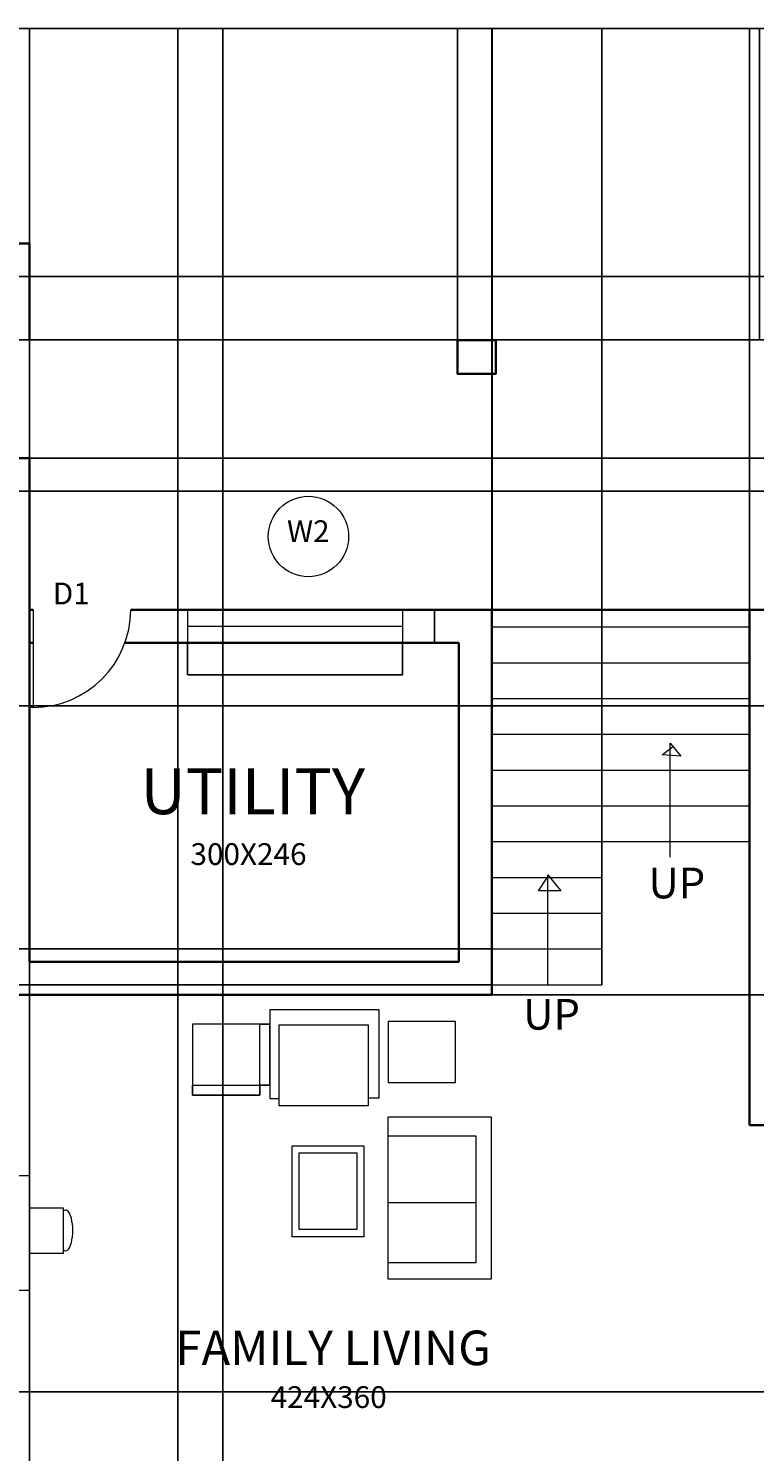
# Model space of a CAD drawing. Units: millimetres. Extents: x -2968 to 14333, y -2966 to 13411.
# Tile 2 of 3: x 3229 to 8301, y 3466 to 13411. Entities that reach past the tile are written whole.
import ezdxf

# ---------------------------------------------------------------- set-up
doc = ezdxf.new("R2010")
doc.units = ezdxf.units.MM
doc.header["$MEASUREMENT"] = 0
for name, color, linetype, lineweight in [('A-ANNO-DIMS', 2, 'Continuous', 18), ('A-ANNO-SYMB', 3, 'Continuous', 13), ('A-ANNO-TEXT', 7, 'Continuous', 18), ('A-AREA-IDEN', 7, 'Continuous', 18), ('A-COLS', 7, 'Continuous', 35), ('A-DOOR', 3, 'Continuous', 18), ('A-FLOR-EDGE', 7, 'Continuous', 25), ('A-FLOR-STRS', 7, 'Continuous', 18), ('A-FURN', 8, 'Continuous', 18), ('A-GLAZ', 4, 'Continuous', 18), ('A-WALL', 7, 'Continuous', 35)]:
    doc.layers.add(name, color=color, linetype=linetype, lineweight=lineweight)
doc.styles.get("Standard").update_dxf_attribs({"font": 'arial.ttf'})
doc.dimstyles.get("Standard").update_dxf_attribs({"dimtxt": 0.18, "dimasz": 0.18, "dimexe": 0.18, "dimexo": 0.0625, "dimgap": 0.09, "dimtad": 0, "dimtih": 1, "dimtoh": 1, "dimdec": 4, "dimzin": 0, "dimdsep": 46, "dimtxsty": 'Standard', "dimcen": 0.09, "dimadec": 0, "dimazin": 0, "dimtfac": 1, "dimtdec": 4, "dimtofl": 0, "dimtmove": 0, "dimatfit": 3, "dimfxl": 1, "dimtolj": 1, "dimtzin": 0, "dimarcsym": 0})

# ---------------------------------------------------------------- blocks, each defined once
blk = doc.blocks.new('WIN-1500')
for p, q in [((-0.0001454069465439, 230.0001364428754), (-0.0001454069465439, 0.0001364428753732)), ((1499.999854593053, 230.0001364428754), (1499.999854593053, 0.0001364428753732)), ((-0.0001454069465439, 115.0001364428753), (1499.999854593053, 115.0001364428753))]:
    blk.add_line(p, q)
blk = doc.blocks.new('DINING-CHAIR')
blk.add_lwpolyline([(8.40971169964e-05, 318.4642751495176), (234.8798944680875, 318.4642751495176), (234.8798944680875, -0.0002547686981416), (8.40971169964e-05, -0.0002547686981416)], close=True)
blk.add_ellipse((251.6572223520761, 161.1385219065178), major_axis=(0, 142.4711695614969), ratio=0.3529417904011299, start_param=2.801418553469442, end_param=6.623359407299936)
blk = doc.blocks.new('VERANDAH-POST')
blk.add_lwpolyline([(-5.84108229305e-05, 235.3216454025205), (266.2404368537072, 235.3216454025205), (266.2404368537072, -0.0003482651118247), (-5.84108229305e-05, -0.0003482651118247)], close=True)
blk = doc.blocks.new('END-TABLE')
blk.add_lwpolyline([(470.3905178718432, 425.6120167429653), (-0.0001639190431888, 425.6120167429653), (-0.0001639190431888, -0.0003055184752156), (470.3905178718432, -0.0003055184752156)], close=True)
blk = doc.blocks.new('*D16')
at = {"layer": 'A-ANNO-DIMS', "color": 0, "lineweight": -2, "transparency": 16777216}
for p, q in [((4341.04331944906, 9117.637743151285), (4341.04331944906, 8892.520243151284)), ((5841.04331944906, 9117.637743151285), (5841.04331944906, 8892.520243151284)), ((4341.223319449061, 8892.700243151285), (5089.785099803767, 8892.700243151285)), ((5840.863319449059, 8892.700243151285), (5092.301539094354, 8892.700243151285))]:
    blk.add_line(p, q, dxfattribs=at)
at = {"layer": 'A-ANNO-DIMS', "color": 0, "transparency": 16777216}
for points in [[(4341.223319449061, 8892.730243151285), (4341.223319449061, 8892.670243151284), (4341.04331944906, 8892.700243151285)], [(5840.863319449059, 8892.730243151285), (5840.863319449059, 8892.670243151284), (5841.04331944906, 8892.700243151285)]]:
    blk.add_solid(points, dxfattribs=at)
at = {"layer": 'Defpoints', "color": 0, "transparency": 16777216}
for p in [(4341.04331944906, 9117.700243151285), (5841.04331944906, 9117.700243151285), (5841.04331944906, 8892.700243151285)]:
    blk.add_point(p, dxfattribs=at)
at = {"layer": 'A-ANNO-DIMS', "color": 0, "transparency": 16777216, "insert": (5091.04331944906, 8892.700243151285), "char_height": 0.18, "attachment_point": 5}
blk.add_mtext('\\A1;WINDOW 1500 TYP.', dxfattribs=at)
blk = doc.blocks.new('*D17')
at = {"layer": 'A-ANNO-DIMS', "color": 0, "lineweight": -2, "transparency": 16777216}
for p, q in [((5841.105819449062, 9347.700243151288), (6066.223319449064, 9347.700243151288)), ((6066.043319449064, 9347.520243151288), (6066.043319449064, 9232.88220768062)), ((6066.043319449064, 9117.880243151289), (6066.043319449064, 9232.518278621958)), ((5841.105819449062, 9117.700243151288), (6066.223319449064, 9117.700243151288))]:
    blk.add_line(p, q, dxfattribs=at)
at = {"layer": 'A-ANNO-DIMS', "color": 0, "transparency": 16777216}
for points in [[(6066.013319449064, 9347.520243151288), (6066.073319449063, 9347.520243151288), (6066.043319449064, 9347.700243151288)], [(6066.013319449064, 9117.880243151289), (6066.073319449063, 9117.880243151289), (6066.043319449064, 9117.700243151288)]]:
    blk.add_solid(points, dxfattribs=at)
at = {"layer": 'Defpoints', "color": 0, "transparency": 16777216}
for p in [(5841.043319449061, 9347.700243151288), (6066.043319449064, 9347.700243151288), (5841.043319449061, 9117.700243151288)]:
    blk.add_point(p, dxfattribs=at)
at = {"layer": 'A-ANNO-DIMS', "color": 0, "transparency": 16777216, "insert": (6066.043319449065, 9232.700243151285), "char_height": 0.18, "attachment_point": 5}
blk.add_mtext('\\A1;230 TYP.', dxfattribs=at)
blk = doc.blocks.new('*D22')
at = {"layer": 'A-ANNO-DIMS', "color": 0, "lineweight": -2, "transparency": 16777216}
for p, q in [((4375.117836080957, 6026.510194481525), (4375.117836080957, 5955.834092212892)), ((4845.508517871843, 6026.510194481525), (4845.508517871843, 5955.834092212892)), ((4375.297836080958, 5956.014092212893), (4608.986260196046, 5956.014092212893)), ((4845.328517871843, 5956.014092212893), (4611.640093756755, 5956.014092212893))]:
    blk.add_line(p, q, dxfattribs=at)
at = {"layer": 'A-ANNO-DIMS', "color": 0, "transparency": 16777216}
for points in [[(4375.297836080958, 5956.044092212891), (4375.297836080958, 5955.984092212893), (4375.117836080957, 5956.014092212893)], [(4845.328517871843, 5956.044092212891), (4845.328517871843, 5955.984092212893), (4845.508517871843, 5956.014092212893)]]:
    blk.add_solid(points, dxfattribs=at)
at = {"layer": 'Defpoints', "color": 0, "transparency": 16777216}
for p in [(4375.117836080957, 6026.572694481525), (4845.508517871843, 6026.572694481525), (4845.508517871843, 5956.014092212893)]:
    blk.add_point(p, dxfattribs=at)
at = {"layer": 'A-ANNO-DIMS', "color": 0, "transparency": 16777216, "insert": (4610.3131769764, 5956.014092212893), "char_height": 0.18, "attachment_point": 5}
blk.add_mtext('\\A1;END TABLE 470 TYP.', dxfattribs=at)
blk = doc.blocks.new('*D23')
at = {"layer": 'A-ANNO-DIMS', "color": 0, "lineweight": -2, "transparency": 16777216}
for p, q in [((4845.571017871845, 6452.185016742969), (4916.24712014048, 6452.185016742969)), ((4916.06712014048, 6452.005016742969), (4916.06712014048, 6239.560758750037)), ((4916.067120140481, 6026.752694481527), (4916.06712014048, 6239.196952474458)), ((4845.571017871845, 6026.572694481527), (4916.247120140481, 6026.572694481527))]:
    blk.add_line(p, q, dxfattribs=at)
at = {"layer": 'A-ANNO-DIMS', "color": 0, "transparency": 16777216}
for points in [[(4916.03712014048, 6452.005016742969), (4916.09712014048, 6452.005016742969), (4916.06712014048, 6452.185016742969)], [(4916.037120140481, 6026.752694481527), (4916.097120140481, 6026.752694481527), (4916.067120140481, 6026.572694481527)]]:
    blk.add_solid(points, dxfattribs=at)
at = {"layer": 'Defpoints', "color": 0, "transparency": 16777216}
for p in [(4845.508517871845, 6452.185016742969), (4916.06712014048, 6452.185016742969), (4845.508517871845, 6026.572694481527)]:
    blk.add_point(p, dxfattribs=at)
at = {"layer": 'A-ANNO-DIMS', "color": 0, "transparency": 16777216, "insert": (4916.067120140481, 6239.378855612245), "char_height": 0.18, "attachment_point": 5}
blk.add_mtext('\\A1;426 TYP.', dxfattribs=at)
blk = doc.blocks.new('*D32')
at = {"layer": 'A-ANNO-DIMS', "color": 0, "lineweight": -2, "transparency": 16777216}
for p, q in [((-1494.810979, 11907.569973), (-1494.810979, 13410.507299)), ((-1494.630979, 13410.327299), (5659.769102855388, 13410.327299)), ((12815.009021, 13410.327299), (5660.608939144611, 13410.327299)), ((12815.189021, 11235.596939), (12815.189021, 13410.507299))]:
    blk.add_line(p, q, dxfattribs=at)
at = {"layer": 'A-ANNO-DIMS', "color": 0, "transparency": 16777216}
for points in [[(-1494.630979, 13410.357299), (-1494.630979, 13410.297299), (-1494.810979, 13410.327299)], [(12815.009021, 13410.357299), (12815.009021, 13410.297299), (12815.189021, 13410.327299)]]:
    blk.add_solid(points, dxfattribs=at)
at = {"layer": 'Defpoints', "color": 0, "transparency": 16777216}
for p in [(12815.189021, 13410.327299), (-1494.810979, 11907.507473), (12815.189021, 11235.534439)]:
    blk.add_point(p, dxfattribs=at)
at = {"layer": 'A-ANNO-DIMS', "color": 0, "transparency": 16777216, "insert": (5660.189021, 13410.327299), "char_height": 0.18, "attachment_point": 5}
blk.add_mtext('\\A1;14310', dxfattribs=at)
blk = doc.blocks.new('*D43')
at = {"layer": 'A-ANNO-DIMS', "color": 0, "lineweight": -2, "transparency": 16777216}
for p, q in [((6465.189021, 9347.569973), (6465.189021, 13410.507299)), ((6465.369021, 13410.327299), (7364.839027821282, 13410.327299)), ((8265.009021, 13410.327299), (7365.539014178718, 13410.327299)), ((8265.189021, 9347.569973), (8265.189021, 13410.507299))]:
    blk.add_line(p, q, dxfattribs=at)
at = {"layer": 'A-ANNO-DIMS', "color": 0, "transparency": 16777216}
for points in [[(6465.369021, 13410.357299), (6465.369021, 13410.297299), (6465.189021, 13410.327299)], [(8265.009021, 13410.357299), (8265.009021, 13410.297299), (8265.189021, 13410.327299)]]:
    blk.add_solid(points, dxfattribs=at)
at = {"layer": 'Defpoints', "color": 0, "transparency": 16777216}
for p in [(8265.189021, 13410.327299), (6465.189021, 9347.507473), (8265.189021, 9347.507473)]:
    blk.add_point(p, dxfattribs=at)
at = {"layer": 'A-ANNO-DIMS', "color": 0, "transparency": 16777216, "insert": (7365.189021, 13410.327299), "char_height": 0.18, "attachment_point": 5}
blk.add_mtext('\\A1;1800', dxfattribs=at)
blk = doc.blocks.new('*D44')
at = {"layer": 'A-ANNO-DIMS', "color": 0, "lineweight": -2, "transparency": 16777216}
for p, q in [((6467.365993, 6728.435381999999), (6467.365993, 13410.507299)), ((6467.545993, 13410.327299), (6850.884355567531, 13410.327299)), ((7235.009021, 13410.327299), (6851.670658432471, 13410.327299)), ((7235.189021, 6728.435381999999), (7235.189021, 13410.507299))]:
    blk.add_line(p, q, dxfattribs=at)
at = {"layer": 'A-ANNO-DIMS', "color": 0, "transparency": 16777216}
for points in [[(6467.545993, 13410.357299), (6467.545993, 13410.297299), (6467.365993, 13410.327299)], [(7235.009021, 13410.357299), (7235.009021, 13410.297299), (7235.189021, 13410.327299)]]:
    blk.add_solid(points, dxfattribs=at)
at = {"layer": 'Defpoints', "color": 0, "transparency": 16777216}
for p in [(7235.189021, 13410.327299), (6467.365993, 6728.372881999999), (7235.189021, 6728.372881999999)]:
    blk.add_point(p, dxfattribs=at)
at = {"layer": 'A-ANNO-DIMS', "color": 0, "transparency": 16777216, "insert": (6851.277507, 13410.327299), "char_height": 0.18, "attachment_point": 5}
blk.add_mtext('\\A1;767.8', dxfattribs=at)
blk = doc.blocks.new('*D45')
at = {"layer": 'A-ANNO-DIMS', "color": 0, "lineweight": -2, "transparency": 16777216}
for p, q in [((6467.303493000004, 6978.372882000003), (-2967.835419000002, 6978.372882000002)), ((-2967.655419000002, 6978.192882000001), (-2967.655419000002, 6853.554785137792)), ((-2967.655419000002, 6728.552882000002), (-2967.655419000002, 6853.190978862212)), ((6467.303493000004, 6728.372882000003), (-2967.835419000002, 6728.372882000002))]:
    blk.add_line(p, q, dxfattribs=at)
at = {"layer": 'A-ANNO-DIMS', "color": 0, "transparency": 16777216}
for points in [[(-2967.685419000002, 6978.192882000001), (-2967.625419000002, 6978.192882000001), (-2967.655419000002, 6978.372882000002)], [(-2967.685419000002, 6728.552882000002), (-2967.625419000002, 6728.552882000002), (-2967.655419000002, 6728.372882000002)]]:
    blk.add_solid(points, dxfattribs=at)
at = {"layer": 'Defpoints', "color": 0, "transparency": 16777216}
for p in [(-2967.655419000002, 6978.372882000002), (6467.365993000004, 6978.372882000003), (6467.365993000004, 6728.372882000003)]:
    blk.add_point(p, dxfattribs=at)
at = {"layer": 'A-ANNO-DIMS', "color": 0, "transparency": 16777216, "insert": (-2967.655419, 6853.372882000001), "char_height": 0.18, "attachment_point": 5}
blk.add_mtext('\\A1;250', dxfattribs=at)
blk = doc.blocks.new('*D47')
at = {"layer": 'A-ANNO-DIMS', "color": 0, "lineweight": -2, "transparency": 16777216}
for p, q in [((-1264.748479, 11677.507473), (14333.28935600001, 11677.507473)), ((14333.10935600001, 11677.327473), (14333.10935600001, 11042.68937613779)), ((14333.10935600001, 10407.687473), (14333.10935600001, 11042.32556986221)), ((-1264.748479, 10407.507473), (14333.28935600001, 10407.507473))]:
    blk.add_line(p, q, dxfattribs=at)
at = {"layer": 'A-ANNO-DIMS', "color": 0, "transparency": 16777216}
for points in [[(14333.07935600001, 11677.327473), (14333.13935600001, 11677.327473), (14333.10935600001, 11677.507473)], [(14333.07935600001, 10407.687473), (14333.13935600001, 10407.687473), (14333.10935600001, 10407.507473)]]:
    blk.add_solid(points, dxfattribs=at)
at = {"layer": 'Defpoints', "color": 0, "transparency": 16777216}
for p in [(-1264.810979000001, 11677.507473), (14333.10935600001, 11677.507473), (-1264.810979000001, 10407.507473)]:
    blk.add_point(p, dxfattribs=at)
at = {"layer": 'A-ANNO-DIMS', "color": 0, "transparency": 16777216, "insert": (14333.10935600001, 11042.507473), "char_height": 0.18, "attachment_point": 5}
blk.add_mtext('\\A1;1270', dxfattribs=at)
blk = doc.blocks.new('*D49')
at = {"layer": 'A-ANNO-DIMS', "color": 0, "lineweight": -2, "transparency": 16777216}
for p, q in [((3235.189021, 232.569973), (3235.189021000001, 13410.507299)), ((3235.369021000001, 13410.327299), (3753.817212416781, 13410.327299)), ((4273.14097, 13410.327299), (3754.69277858322, 13410.327299)), ((4273.320969999999, 232.569973), (4273.320970000001, 13410.507299))]:
    blk.add_line(p, q, dxfattribs=at)
at = {"layer": 'A-ANNO-DIMS', "color": 0, "transparency": 16777216}
for points in [[(3235.369021000001, 13410.357299), (3235.369021000001, 13410.297299), (3235.189021000001, 13410.327299)], [(4273.14097, 13410.357299), (4273.14097, 13410.297299), (4273.320970000001, 13410.327299)]]:
    blk.add_solid(points, dxfattribs=at)
at = {"layer": 'Defpoints', "color": 0, "transparency": 16777216}
for p in [(4273.320970000001, 13410.327299), (3235.189021, 232.507473), (4273.320969999999, 232.507473)]:
    blk.add_point(p, dxfattribs=at)
at = {"layer": 'A-ANNO-DIMS', "color": 0, "transparency": 16777216, "insert": (3754.254995500001, 13410.327299), "char_height": 0.18, "attachment_point": 5}
blk.add_mtext('\\A1;1038.1', dxfattribs=at)
blk = doc.blocks.new('*D50')
at = {"layer": 'A-ANNO-DIMS', "color": 0, "lineweight": -2, "transparency": 16777216}
for p, q in [((3235.189021, 11235.596939), (3235.189021, 13410.507299)), ((3235.369021, 13410.327299), (4730.825595415415, 13410.327299)), ((6227.000942, 13410.327299), (4731.544367584583, 13410.327299)), ((6227.180942, 11232.243145), (6227.180942, 13410.507299))]:
    blk.add_line(p, q, dxfattribs=at)
at = {"layer": 'A-ANNO-DIMS', "color": 0, "transparency": 16777216}
for points in [[(3235.369021, 13410.357299), (3235.369021, 13410.297299), (3235.189021, 13410.327299)], [(6227.000942, 13410.357299), (6227.000942, 13410.297299), (6227.180942, 13410.327299)]]:
    blk.add_solid(points, dxfattribs=at)
at = {"layer": 'Defpoints', "color": 0, "transparency": 16777216}
for p in [(6227.180942, 13410.327299), (3235.189021, 11235.534439), (6227.180942, 11232.180645)]:
    blk.add_point(p, dxfattribs=at)
at = {"layer": 'A-ANNO-DIMS', "color": 0, "transparency": 16777216, "insert": (4731.184981499999, 13410.327299), "char_height": 0.18, "attachment_point": 5}
blk.add_mtext('\\A1;2992', dxfattribs=at)
blk = doc.blocks.new('*D51')
at = {"layer": 'A-ANNO-DIMS', "color": 0, "lineweight": -2, "transparency": 16777216}
for p, q in [((6227.180942, 11232.243145), (6227.180942, 13410.507299)), ((6227.360942, 13410.327299), (7281.505338680763, 13410.327299)), ((8336.57994, 13410.327299), (7282.435543319237, 13410.327299)), ((8336.75994, 11232.243145), (8336.75994, 13410.507299))]:
    blk.add_line(p, q, dxfattribs=at)
at = {"layer": 'A-ANNO-DIMS', "color": 0, "transparency": 16777216}
for points in [[(6227.360942, 13410.357299), (6227.360942, 13410.297299), (6227.180942, 13410.327299)], [(8336.57994, 13410.357299), (8336.57994, 13410.297299), (8336.75994, 13410.327299)]]:
    blk.add_solid(points, dxfattribs=at)
at = {"layer": 'Defpoints', "color": 0, "transparency": 16777216}
for p in [(8336.75994, 13410.327299), (6227.180942, 11232.180645), (8336.75994, 11232.180645)]:
    blk.add_point(p, dxfattribs=at)
at = {"layer": 'A-ANNO-DIMS', "color": 0, "transparency": 16777216, "insert": (7281.970441, 13410.327299), "char_height": 0.18, "attachment_point": 5}
blk.add_mtext('\\A1;2109.6', dxfattribs=at)
blk = doc.blocks.new('*D54')
at = {"layer": 'A-ANNO-DIMS', "color": 0, "lineweight": -2, "transparency": 16777216}
for p, q in [((-1220.345468, 3884.149375000002), (14333.28935600001, 3884.149375000005)), ((14333.10935600001, 3883.969375000005), (14333.10935600001, 2738.596660637794)), ((14333.10935600001, 1592.860140000003), (14333.10935600001, 2738.232854362214)), ((-1220.345468, 1592.680140000001), (14333.28935600001, 1592.680140000003))]:
    blk.add_line(p, q, dxfattribs=at)
at = {"layer": 'A-ANNO-DIMS', "color": 0, "transparency": 16777216}
for points in [[(14333.07935600001, 3883.969375000005), (14333.13935600001, 3883.969375000005), (14333.10935600001, 3884.149375000005)], [(14333.07935600001, 1592.860140000003), (14333.13935600001, 1592.860140000003), (14333.10935600001, 1592.680140000003)]]:
    blk.add_solid(points, dxfattribs=at)
at = {"layer": 'Defpoints', "color": 0, "transparency": 16777216}
for p in [(-1220.407968, 3884.149375000002), (14333.10935600001, 3884.149375000005), (-1220.407968, 1592.680140000001)]:
    blk.add_point(p, dxfattribs=at)
at = {"layer": 'A-ANNO-DIMS', "color": 0, "transparency": 16777216, "insert": (14333.10935600001, 2738.414757499999), "char_height": 0.18, "attachment_point": 5}
blk.add_mtext('\\A1;2291.5', dxfattribs=at)
blk = doc.blocks.new('*D55')
at = {"layer": 'A-ANNO-DIMS', "color": 0, "lineweight": -2, "transparency": 16777216}
for p, q in [((-1494.748479, 6657.507473000004), (14333.28935600001, 6657.507473000006)), ((14333.10935600001, 6657.327473000005), (14333.10935600001, 5271.010388529336)), ((14333.10935600002, 3884.329375000005), (14333.10935600001, 5270.646459470672)), ((-1220.345468, 3884.149375000002), (14333.28935600002, 3884.149375000005))]:
    blk.add_line(p, q, dxfattribs=at)
at = {"layer": 'A-ANNO-DIMS', "color": 0, "transparency": 16777216}
for points in [[(14333.07935600001, 6657.327473000005), (14333.13935600001, 6657.327473000005), (14333.10935600001, 6657.507473000006)], [(14333.07935600002, 3884.329375000005), (14333.13935600001, 3884.329375000005), (14333.10935600002, 3884.149375000005)]]:
    blk.add_solid(points, dxfattribs=at)
at = {"layer": 'Defpoints', "color": 0, "transparency": 16777216}
for p in [(-1494.810979, 6657.507473000004), (14333.10935600001, 6657.507473000006), (-1220.407968, 3884.149375000002)]:
    blk.add_point(p, dxfattribs=at)
at = {"layer": 'A-ANNO-DIMS', "color": 0, "transparency": 16777216, "insert": (14333.10935600001, 5270.828424), "char_height": 0.18, "attachment_point": 5}
blk.add_mtext('\\A1;2773.4', dxfattribs=at)
blk = doc.blocks.new('*D57')
at = {"layer": 'A-ANNO-DIMS', "color": 0, "lineweight": -2, "transparency": 16777216}
for p, q in [((1665.064982, -1259.254558), (1665.064982000001, 13410.507299)), ((1665.244982000001, 13410.327299), (3125.078715848568, 13410.327299)), ((4585.598316000001, 13410.327299), (3125.764582151433, 13410.327299)), ((4585.778315999999, -1259.254558), (4585.778316000001, 13410.507299))]:
    blk.add_line(p, q, dxfattribs=at)
at = {"layer": 'A-ANNO-DIMS', "color": 0, "transparency": 16777216}
for points in [[(1665.244982000001, 13410.357299), (1665.244982000001, 13410.297299), (1665.064982000001, 13410.327299)], [(4585.598316000001, 13410.357299), (4585.598316000001, 13410.297299), (4585.778316000001, 13410.327299)]]:
    blk.add_solid(points, dxfattribs=at)
at = {"layer": 'Defpoints', "color": 0, "transparency": 16777216}
for p in [(4585.778316000001, 13410.327299), (1665.064982, -1259.317058), (4585.778315999999, -1259.317058)]:
    blk.add_point(p, dxfattribs=at)
at = {"layer": 'A-ANNO-DIMS', "color": 0, "transparency": 16777216, "insert": (3125.421649000001, 13410.327299), "char_height": 0.18, "attachment_point": 5}
blk.add_mtext('\\A1;2921', dxfattribs=at)
blk = doc.blocks.new('*D61')
at = {"layer": 'A-ANNO-DIMS', "color": 0, "lineweight": -2, "transparency": 16777216}
for p, q in [((1505.251521, 10177.507473), (14333.28935600001, 10177.507473)), ((14333.10935600001, 10177.327473), (14333.10935600001, 9427.689376137798)), ((14333.10935600001, 8677.687473000007), (14333.10935600001, 9427.325569862218)), ((1505.251521, 8677.507473000003), (14333.28935600001, 8677.507473000007))]:
    blk.add_line(p, q, dxfattribs=at)
at = {"layer": 'A-ANNO-DIMS', "color": 0, "transparency": 16777216}
for points in [[(14333.07935600001, 10177.327473), (14333.13935600001, 10177.327473), (14333.10935600001, 10177.507473)], [(14333.07935600001, 8677.687473000007), (14333.13935600001, 8677.687473000007), (14333.10935600001, 8677.507473000007)]]:
    blk.add_solid(points, dxfattribs=at)
at = {"layer": 'Defpoints', "color": 0, "transparency": 16777216}
for p in [(1505.189021, 10177.507473), (14333.10935600001, 10177.507473), (1505.189021, 8677.507473000003)]:
    blk.add_point(p, dxfattribs=at)
at = {"layer": 'A-ANNO-DIMS', "color": 0, "transparency": 16777216, "insert": (14333.10935600001, 9427.507473000001), "char_height": 0.18, "attachment_point": 5}
blk.add_mtext('\\A1;1500', dxfattribs=at)

msp = doc.modelspace()

# ---------------------------------------------------------------- linework, layer by layer
at = {"layer": 'A-ANNO-SYMB'}
for points in [[(7712.199242320145, 7618.934004650917), (7712.199242320145, 8415.524808817892), (7785.424564020941, 8326.111813228461), (7655.246677664807, 8334.240447608754), (7728.471999365604, 8391.13940132549)], [(6857.902432476404, 6732.929709246033), (6857.902432476404, 7497.006967188733), (6947.400511222426, 7383.208068458421), (6792.812794297235, 7383.208068458421), (6849.765358952573, 7472.621559696271)]]:
    msp.add_lwpolyline(points, dxfattribs=at)
msp.add_circle((5184.743742056191, 9860.213910516351), 280.7929963504647, dxfattribs=at)
at = {"layer": 'A-DOOR'}
msp.add_lwpolyline([(3261.29201869457, 9347.836903303887), (3261.29201869457, 8666.348579443365), (3233.993676473896, 8666.348579443365), (3233.993676473896, 9347.836903303887)], close=True, dxfattribs=at)
msp.add_arc((3261.29201869457, 9347.836903303887), 681.7287306783696, 270, 0, dxfattribs=at)
at = {"layer": 'A-FLOR-EDGE'}
msp.add_line((3005.189021442665, 11235.53443915362), (12815.18902144266, 11235.53443915362), dxfattribs=at)
at = {"layer": 'A-FLOR-STRS'}
for p, q in [((7235.189021442668, 6728.372881745513), (7235.189021442664, 9347.507473364632)), ((6467.365993403596, 9228.372881745512), (8265.45908183977, 9228.372881745512)), ((6467.365993403596, 8978.372881745512), (8265.45908183977, 8978.372881745512)), ((6467.365993403596, 8728.372881745512), (8265.45908183977, 8728.372881745512)), ((6467.365993403596, 8478.372881745512), (8265.45908183977, 8478.372881745512)), ((6467.365993403596, 8228.372881745512), (8265.45908183977, 8228.372881745512)), ((6467.365993403596, 7978.372881745513), (8265.45908183977, 7978.372881745513)), ((6467.365993403596, 7728.372881745513), (8265.45908183977, 7728.372881745513)), ((6467.365993403596, 7478.372881745513), (7235.189021442668, 7478.372881745513)), ((8265.189021442662, 7478.372881745513), (8265.45908183977, 7478.372881745513)), ((6467.365993403596, 7228.372881745513), (7235.189021442668, 7228.372881745513)), ((8265.189021442662, 7228.372881745513), (8265.45908183977, 7228.372881745513)), ((6467.365993403596, 6978.372881745513), (7235.189021442668, 6978.372881745513)), ((8265.189021442662, 6978.372881745513), (8265.45908183977, 6978.372881745513)), ((6467.365993403596, 6728.372881745513), (7235.189021442668, 6728.372881745513)), ((8265.189021442662, 6728.372881745511), (8265.45908183977, 6728.372881745513))]:
    msp.add_line(p, q, dxfattribs=at)
at = {"layer": 'A-FURN'}
msp.add_line((5741.930737728253, 5207.03832412773), (6355.116356844548, 5207.03832412773), dxfattribs=at)
for points in [[(5602.331415713532, 5937.838241603458), (5679.990844783839, 5937.838241603458), (5679.990844783839, 6552.981074355485), (4914.495722528547, 6552.981074355485), (4914.495722528547, 5932.296396420163), (4981.060153158847, 5932.296396420163)], [(5741.915447702631, 5671.896089695977), (6354.311545506818, 5671.896089695977), (6354.311545506818, 4785.203834259358), (5741.915447702631, 4785.203834259358)]]:
    msp.add_lwpolyline(points, dxfattribs=at)
for points in [[(4981.060153158847, 6447.686511521286), (5602.331415713532, 6447.686511521286), (5602.331415713532, 5882.420285418921), (4981.060153158847, 5882.420285418921)], [(5741.915447702631, 5804.899878446595), (6460.814912515693, 5804.899878446595), (6460.814912515693, 4669.933850965579), (5741.915447702631, 4669.933850965579)], [(5070.613831997383, 5602.638637830562), (5572.326825845987, 5602.638637830562), (5572.326825845987, 4966.451068057039), (5070.613831997383, 4966.451068057039)], [(5120.613831997383, 5552.638637830561), (5522.326825845986, 5552.638637830561), (5522.326825845986, 5016.451068057039), (5120.613831997383, 5016.451068057039)], [(627.8926181816496, 5394.823160820234), (3236.742084097117, 5394.823160820234), (3236.742084097117, 4590.28017311683), (627.8926181816496, 4590.28017311683)]]:
    msp.add_lwpolyline(points, close=True, dxfattribs=at)
at = {"layer": 'A-WALL'}
for p, q in [((-1494.810978557335, 11907.50747336463), (3235.189021442665, 11907.50747336463)), ((3235.189021442665, 11235.53443915362), (3235.189021442665, 11907.50747336463)), ((1245.636054873233, 10407.50747336463), (3235.189021442665, 10407.50747336463)), ((3235.189021442665, 9347.507473364634), (3235.189021442665, 10407.50747336463)), ((3235.189021442665, 9347.507473364634), (3261.29201869457, 9347.507473364634)), ((3235.189021442665, 6887.507473364634), (3235.189021442665, 9347.507473364634)), ((3943.020669778164, 9347.507473364634), (12815.18902144266, 9347.507473364634)), ((6465.189021442665, 6657.507473364635), (6465.189021442665, 9347.507473364634)), ((8265.189021442662, 5747.507473364635), (8265.189021442662, 9347.507473364634)), ((3235.189021442665, 9117.507473364634), (3261.29201869457, 9117.507473364634)), ((3902.932428843588, 9117.507473364632), (6235.189021442665, 9117.507473364632)), ((6235.189021442666, 6887.507473364634), (6235.189021442665, 9117.507473364634)), ((3235.189021442665, 6887.507473364634), (6235.189021442664, 6887.507473364634)), ((1390.189021442665, 6657.507473364633), (6465.189021442665, 6657.507473364635)), ((8265.189021442662, 5747.507473364635), (8495.189021442664, 5747.507473364635))]:
    msp.add_line(p, q, dxfattribs=at)

# ---------------------------------------------------------------- block references
at = {"layer": 'A-COLS'}
msp.add_blockref('VERANDAH-POST', (6227.180999999999, 10996.859), dxfattribs=at)
at = {"layer": 'A-FURN'}
for name, p in [('END-TABLE', (5741.915611621674, 6044.306805456839)), ('END-TABLE', (4375.118, 6026.573)), ('DINING-CHAIR', (3236.742, 4850.081))]:
    msp.add_blockref(name, p, dxfattribs=at)
at = {"layer": 'A-GLAZ'}
msp.add_blockref('WIN-1500', (4341.043464856007, 9117.70010670841), dxfattribs=at)

# ---------------------------------------------------------------- texts
at = {"layer": 'A-ANNO-SYMB'}
for s, p in [('W2', (5034.941835008561, 9821.047556128355)), ('D1', (3398.988753154874, 9385.618741903456))]:
    msp.add_text(s, height=152.3112078732942, dxfattribs=at).set_placement(p)
at = {"layer": 'A-ANNO-TEXT'}
for p in [(7560.193046432591, 7331.623975824536), (6685.026741903644, 6414.084048563179)]:
    msp.add_text('UP', height=214.6542409740552, dxfattribs=at).set_placement(p)
at = {"layer": 'A-AREA-IDEN'}
for s, height, p in [('UTILITY', 321.4922915585339, (4011.699140124022, 7919.665711171925)), ('300X246', 152.3112078732942, (4360.770013935257, 7564.772043656851)), ('FAMILY LIVING', 241.7589680836474, (4255.389284688258, 4069.542678558383)), ('424X360', 152.3112078732942, (4920.680375463655, 3770.169810176188))]:
    msp.add_text(s, height=height, dxfattribs=at).set_placement(p)

# ---------------------------------------------------------------- dimensions: what is measured, and where the dimension line sits
at = {"layer": 'A-ANNO-DIMS'}
for base, p1, p2, override, picture, middle in [((12815.189021, 13410.327299), (-1494.810979, 11907.507473), (12815.189021, 11235.534439), {"dimdec": 0, "dimlfac": 1, "dimrnd": 0, "dimzin": 0, "dimdsep": 46, "dimlunit": 2}, '*D32', (5660.189021, 13410.327299)), ((4585.778316000001, 13410.327299), (1665.064982, -1259.317058), (4585.778315999999, -1259.317058), {"dimdec": 0, "dimlfac": 1, "dimrnd": 0, "dimzin": 0, "dimdsep": 46, "dimlunit": 2}, '*D57', (3125.421649000001, 13410.327299)), ((4273.320970000001, 13410.327299), (3235.189021, 232.507473), (4273.320969999999, 232.507473), {"dimdec": 1, "dimlfac": 1, "dimrnd": 0, "dimzin": 0, "dimdsep": 46, "dimlunit": 2}, '*D49', (3754.254995500001, 13410.327299)), ((6227.180942, 13410.327299), (3235.189021, 11235.534439), (6227.180942, 11232.180645), {"dimdec": 0, "dimlfac": 1, "dimrnd": 0, "dimzin": 0, "dimdsep": 46, "dimlunit": 2}, '*D50', (4731.184981499999, 13410.327299)), ((8336.75994, 13410.327299), (6227.180942, 11232.180645), (8336.75994, 11232.180645), {"dimdec": 1, "dimlfac": 1, "dimrnd": 0, "dimzin": 0, "dimdsep": 46, "dimlunit": 2}, '*D51', (7281.970441, 13410.327299)), ((8265.189021, 13410.327299), (6465.189021, 9347.507473), (8265.189021, 9347.507473), {"dimdec": 0, "dimlfac": 1, "dimrnd": 0, "dimzin": 0, "dimdsep": 46, "dimlunit": 2}, '*D43', (7365.189021, 13410.327299)), ((7235.189021, 13410.327299), (6467.365993, 6728.372881999999), (7235.189021, 6728.372881999999), {"dimdec": 1, "dimlfac": 1, "dimrnd": 0, "dimzin": 0, "dimdsep": 46, "dimlunit": 2}, '*D44', (6851.277507, 13410.327299))]:
    dim = msp.add_linear_dim(base=base, p1=p1, p2=p2, dimstyle='Standard', override=override, dxfattribs=at)
    dim.commit()
    dim.dimension.update_dxf_attribs({"geometry": picture, "text_midpoint": middle})
for base, p1, p2, override, picture, middle in [((14333.10935600001, 11677.507473), (-1264.810979, 10407.507473), (-1264.810979, 11677.507473), {"dimdec": 0, "dimlfac": 1, "dimrnd": 0, "dimzin": 0, "dimdsep": 46, "dimlunit": 2}, '*D47', (14333.10935600001, 11042.507473)), ((14333.10935600001, 10177.507473), (1505.189021, 8677.507473), (1505.189021, 10177.507473), {"dimdec": 0, "dimlfac": 1, "dimrnd": 0, "dimzin": 0, "dimdsep": 46, "dimlunit": 2}, '*D61', (14333.10935600001, 9427.507473000001)), ((-2967.655419000002, 6978.372882000002), (6467.365993, 6728.372881999999), (6467.365993, 6978.372881999999), {"dimdec": 0, "dimlfac": 1, "dimrnd": 0, "dimzin": 0, "dimdsep": 46, "dimlunit": 2}, '*D45', (-2967.655419, 6853.372882000001)), ((14333.10935600001, 6657.507473000006), (-1220.407968, 3884.149375), (-1494.810979, 6657.507472999999), {"dimdec": 1, "dimlfac": 1, "dimrnd": 0, "dimzin": 0, "dimdsep": 46, "dimlunit": 2}, '*D55', (14333.10935600001, 5270.828424)), ((14333.10935600001, 3884.149375000005), (-1220.407968, 1592.68014), (-1220.407968, 3884.149375), {"dimdec": 1, "dimlfac": 1, "dimrnd": 0, "dimzin": 0, "dimdsep": 46, "dimlunit": 2}, '*D54', (14333.10935600001, 2738.414757499999))]:
    dim = msp.add_linear_dim(base=base, p1=p1, p2=p2, angle=90, dimstyle='Standard', override=override, dxfattribs=at)
    dim.commit()
    dim.dimension.update_dxf_attribs({"geometry": picture, "text_midpoint": middle})
for base, p1, p2, picture, middle in [((6066.043319449064, 9347.700243151288), (5841.04331944906, 9117.700243151285), (5841.04331944906, 9347.700243151285), '*D17', (6066.043319449065, 9232.700243151285)), ((4916.06712014048, 6452.185016742969), (4845.508517871843, 6026.572694481525), (4845.508517871843, 6452.185016742966), '*D23', (4916.067120140481, 6239.378855612245))]:
    dim = msp.add_linear_dim(base=base, p1=p1, p2=p2, angle=90, text='<> TYP.', dimstyle='Standard', override={"dimdec": 0, "dimlfac": 1, "dimrnd": 0, "dimzin": 0, "dimdsep": 46, "dimlunit": 2}, dxfattribs=at)
    dim.commit()
    dim.dimension.update_dxf_attribs({"geometry": picture, "text_midpoint": middle})
for base, p1, p2, text, picture, middle in [((5841.04331944906, 8892.700243151285), (4341.04331944906, 9117.700243151285), (5841.04331944906, 9117.700243151285), 'WINDOW <> TYP.', '*D16', (5091.04331944906, 8892.700243151285)), ((4845.508517871843, 5956.014092212893), (4375.117836080957, 6026.572694481525), (4845.508517871843, 6026.572694481525), 'END TABLE <> TYP.', '*D22', (4610.3131769764, 5956.014092212893))]:
    dim = msp.add_linear_dim(base=base, p1=p1, p2=p2, text=text, dimstyle='Standard', override={"dimdec": 0, "dimlfac": 1, "dimrnd": 0, "dimzin": 0, "dimdsep": 46, "dimlunit": 2}, dxfattribs=at)
    dim.commit()
    dim.dimension.update_dxf_attribs({"geometry": picture, "text_midpoint": middle})

doc.saveas('drawing.dxf')
